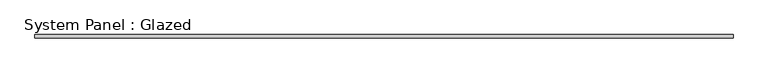
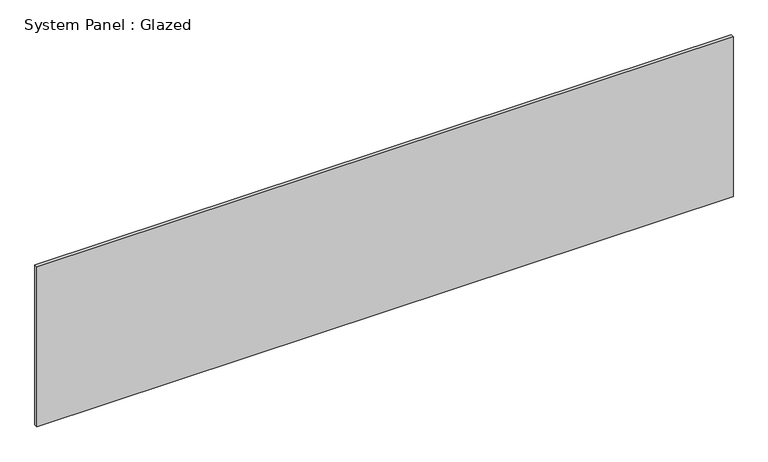
"""IFC4 building model written with IfcOpenShell, lengths in millimetres: plate geometry, System Panel : Glazed."""

from ifc_helpers import new_model, si_unit, origin, origin_with_axes, place, context, project, spatial, polyline, outline, extrude, source, transform, mapped, element, save


def system_panel_glazed_a39085c9(model_context):
    return source(origin(), model_context, "Body", "SweptSolid", [
        extrude(outline(polyline([(2513.2718784, 19.05), (-2513.2718784, 19.05), (-2513.2718784, 44.45), (2513.2718784, 44.45), (2513.2718784, 19.05)])), origin_with_axes(), (0.0, 0.0, 1.0), 1219.2),
    ])


if __name__ == "__main__":
    model = new_model("IFC4")
    model_context = context("Model", 3, world=origin())
    ifc_project = project(units=[si_unit("LENGTHUNIT", "METRE", prefix="MILLI")], contexts=[model_context])
    site = spatial("IfcSite", under=ifc_project)
    building = spatial("IfcBuilding", under=site)
    placement = place(None, origin())
    system_panel_glazed_shape = system_panel_glazed_a39085c9(model_context)
    element("IfcPlate", 1, ObjectType="System Panel : Glazed", at=placement, inside=building, context=model_context, shape_type="MappedRepresentation", body=[
        mapped(system_panel_glazed_shape, transform((0.0, 0.0, 0.0), x_axis=(1.0, 0.0, 0.0), y_axis=(0.0, 1.0, 0.0), z_axis=(0.0, 0.0, 1.0))),
    ])
    save(model, "model.ifc")

# Revit data of these elements
# Type "System Panel : Glazed"
#   Construction Type Id = "GSP4R"
#   Analytic Construction = "1/8 in Pilkington single glazing"
#   Visual Light Transmittance = 0.9
#   Solar Heat Gain Coefficient = 0.86
#   Heat Transfer Coefficient (U) = 1.18115 BTU/(h·ft²·°F)
# Element 1 (IfcPlate, "System Panel : Glazed")
#   Materials on its faces: "Glass"
# Materials
#   "Glass": class "Glass", colour RGB 0 128 192, transparency 0.75, Description = "Soda Lime Glass", Cost = 0
